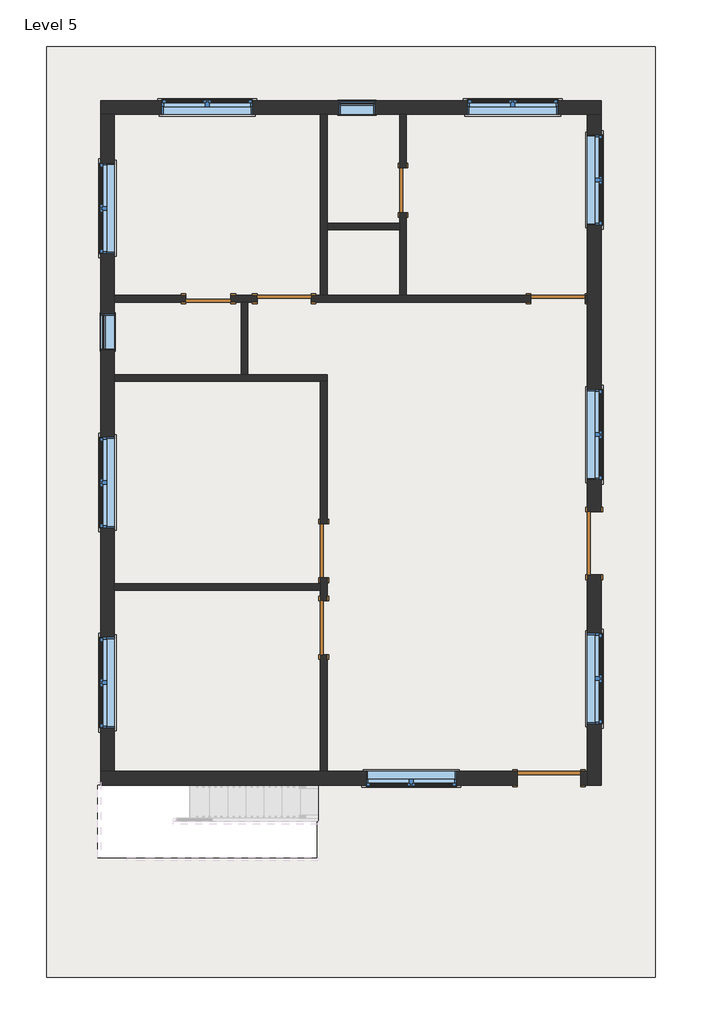
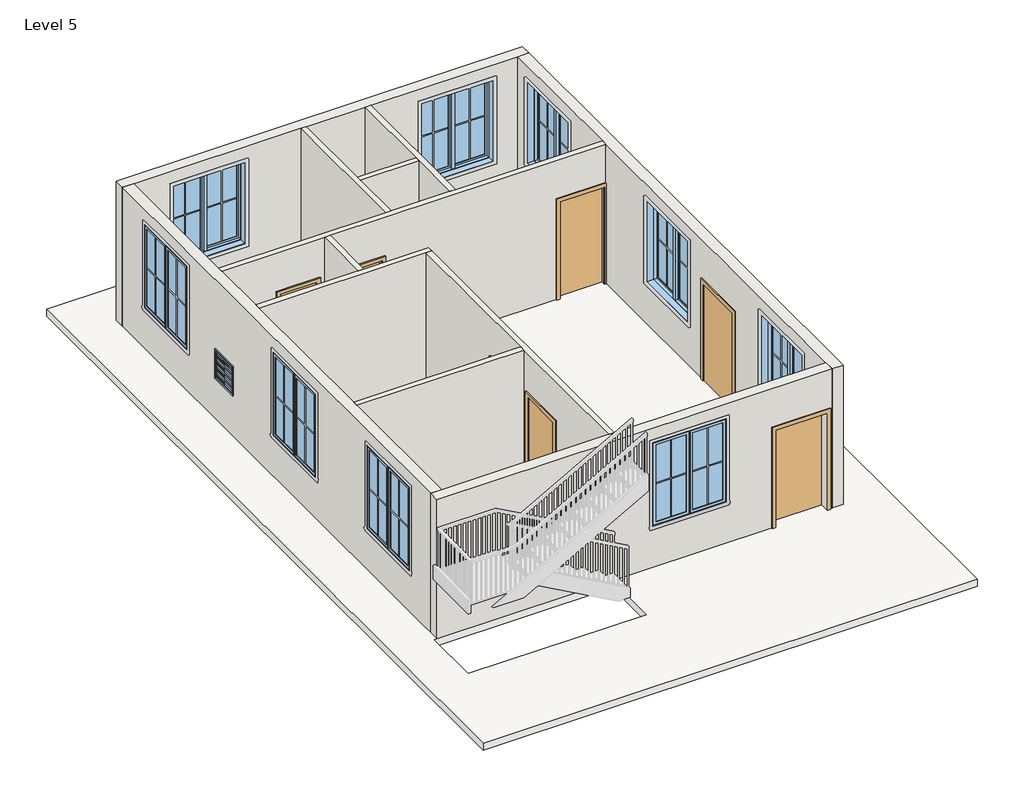
# One storey, part 1 of 3: 12 walls, 11 windows, 8 doors, 1 roof.
"""IFC4 building model written with IfcOpenShell, lengths in millimetres."""

from ifc_helpers import new_model, si_unit, frame, origin, place, context, project, spatial, polyline, outline, extrude, faceted_brep, transform, mapped, element, save
from components import door_78caadf7, single_flush_door_3_e5f9f3c4, single_flush_door_3_305aa2a5, door_9d399b00, door_0848dd25, window_casement_double_win_5_f93960c7, window_f2d8fef0

model = new_model("IFC4")

# Units and contexts
model_context = context("Model", 3, world=origin())
ifc_project = project(units=[si_unit("LENGTHUNIT", "METRE", prefix="MILLI")], contexts=[model_context])

# Site, building, storey
site = spatial("IfcSite", under=ifc_project)
building = spatial("IfcBuilding", under=site)
storey = spatial("IfcBuildingStorey", under=building, Name="Level 5", Elevation=9601.2)

# Doors
placement = place(None, origin())
door_shape = door_78caadf7(model_context)
element("IfcDoor", 1, ObjectType="Single-Flush : DOOR 2'6\"", at=placement, inside=storey, context=model_context, shape_type="MappedRepresentation", body=[
    mapped(door_shape, transform((-377.1698569, 4707.5566963, 9601.2), x_axis=(0.0, -1.0, 0.0), y_axis=(1.0, 0.0, 0.0), z_axis=(0.0, 0.0, 1.0))),
])
element("IfcDoor", 2, ObjectType="Single-Flush : DOOR 2'6\"", at=placement, inside=storey, context=model_context, shape_type="MappedRepresentation", body=[
    mapped(door_shape, transform((-3653.7698569, 2878.7566963, 9601.2), x_axis=(1.0, 0.0, 0.0), y_axis=(0.0, 1.0, 0.0), z_axis=(0.0, 0.0, 1.0))),
])
single_flush_door_3_shape = single_flush_door_3_e5f9f3c4(model_context)
element("IfcDoor", 3, ObjectType="Single-Flush : DOOR 3'", at=placement, inside=storey, context=model_context, shape_type="MappedRepresentation", body=[
    mapped(single_flush_door_3_shape, transform((-2377.4198569, 2878.7566963, 9601.2), x_axis=(1.0, 0.0, 0.0), y_axis=(0.0, 1.0, 0.0), z_axis=(0.0, 0.0, 1.0))),
])
element("IfcDoor", 4, ObjectType="Single-Flush : DOOR 3'", at=placement, inside=storey, context=model_context, shape_type="MappedRepresentation", body=[
    mapped(single_flush_door_3_shape, transform((2232.6801431, 2878.7566963, 9601.2), x_axis=(1.0, 0.0, 0.0), y_axis=(0.0, 1.0, 0.0), z_axis=(0.0, 0.0, 1.0))),
])
element("IfcDoor", 5, ObjectType="Single-Flush : DOOR 3'", at=placement, inside=storey, context=model_context, shape_type="MappedRepresentation", body=[
    mapped(single_flush_door_3_shape, transform((-1710.6698569, -2658.4433037, 9601.2), x_axis=(0.0, 1.0, 0.0), y_axis=(-1.0, 0.0, 0.0), z_axis=(0.0, 0.0, 1.0))),
])
single_flush_door_3_2_shape = single_flush_door_3_305aa2a5(model_context)
element("IfcDoor", 6, ObjectType="Single-Flush : DOOR 3'", at=placement, inside=storey, context=model_context, shape_type="MappedRepresentation", body=[
    mapped(single_flush_door_3_2_shape, transform((-1710.6698569, -1363.0433037, 9601.2), x_axis=(0.0, -1.0, 0.0), y_axis=(1.0, 0.0, 0.0), z_axis=(0.0, 0.0, 1.0))),
])
door_2_shape = door_9d399b00(model_context)
element("IfcDoor", 7, ObjectType="Single-Flush : DOOR 3'6\"", at=placement, inside=storey, context=model_context, shape_type="MappedRepresentation", body=[
    mapped(door_2_shape, transform((2080.2801431, -5192.0933037, 9601.2), x_axis=(1.0, 0.0, 0.0), y_axis=(0.0, 1.0, 0.0), z_axis=(0.0, 0.0, 1.0))),
])
door_3_shape = door_0848dd25(model_context)
element("IfcDoor", 8, ObjectType="Single-Flush : DOOR 3'6\"", at=placement, inside=storey, context=model_context, shape_type="MappedRepresentation", body=[
    mapped(door_3_shape, transform((2842.2801431, -1236.0433037, 9601.2), x_axis=(0.0, -1.0, 0.0), y_axis=(1.0, 0.0, 0.0), z_axis=(0.0, 0.0, 1.0))),
])

# Roof
element("IfcRoof", 9, ObjectType="ROOF 6\"", at=placement, inside=storey, context=model_context, shape_type="SweptSolid", body=[
    extrude(outline(polyline([(-6377.9198569, -8544.8933037), (-6377.9198569, 7126.9066963), (3870.9801431, 7126.9066963), (3870.9801431, -8544.8933037), (-6377.9198569, -8544.8933037)]), holes=[polyline([(-5514.3198569, -5306.3933037), (-5514.3198569, -6525.5933037), (-1831.3198569, -6525.5933037), (-1831.3198569, -5306.3933037), (-5514.3198569, -5306.3933037)])]), frame((0.0, 0.0, 9448.8), z_axis=(0.0, 0.0, 1.0), x_axis=(1.0, 0.0, 0.0)), (0.0, 0.0, 1.0), 152.4),
])

# Walls
element("IfcWall", 10, ObjectType="WALL 4.5\"", at=placement, inside=storey, context=model_context, shape_type="Brep", body=[
    faceted_brep([(2689.8801431, 2821.6066963, 11734.8), (2689.8801431, 2821.6066963, 9601.2), (2727.9801431, 2821.6066963, 9601.2), (2727.9801431, 2821.6066963, 12649.2), (-2987.0198569, 2821.6066963, 12649.2), (-3101.3198569, 2821.6066963, 12649.2), (-5234.9198569, 2821.6066963, 12649.2), (-5234.9198569, 2821.6066963, 9601.2), (-4034.7698569, 2821.6066963, 9601.2), (-4034.7698569, 2821.6066963, 11734.8), (-3272.7698569, 2821.6066963, 11734.8), (-3272.7698569, 2821.6066963, 9601.2), (-3101.3198569, 2821.6066963, 9601.2), (-2987.0198569, 2821.6066963, 9601.2), (-2834.6198569, 2821.6066963, 9601.2), (-2834.6198569, 2821.6066963, 11734.8), (-1920.2198569, 2821.6066963, 11734.8), (-1920.2198569, 2821.6066963, 9601.2), (1775.4801431, 2821.6066963, 9601.2), (1775.4801431, 2821.6066963, 11734.8), (2727.9801431, 2935.9066963, 9601.2), (2689.8801431, 2935.9066963, 9601.2), (2689.8801431, 2935.9066963, 11734.8), (1775.4801431, 2935.9066963, 11734.8), (1775.4801431, 2935.9066963, 9601.2), (-320.0198569, 2935.9066963, 9601.2), (-434.3198569, 2935.9066963, 9601.2), (-1653.5198569, 2935.9066963, 9601.2), (-1767.8198569, 2935.9066963, 9601.2), (-1920.2198569, 2935.9066963, 9601.2), (-1920.2198569, 2935.9066963, 11734.8), (-2834.6198569, 2935.9066963, 11734.8), (-2834.6198569, 2935.9066963, 9601.2), (-3272.7698569, 2935.9066963, 9601.2), (-3272.7698569, 2935.9066963, 11734.8), (-4034.7698569, 2935.9066963, 11734.8), (-4034.7698569, 2935.9066963, 9601.2), (-5234.9198569, 2935.9066963, 9601.2), (-5234.9198569, 2935.9066963, 12649.2), (-1767.8198569, 2935.9066963, 12649.2), (-1653.5198569, 2935.9066963, 12649.2), (-434.3198569, 2935.9066963, 12649.2), (-320.0198569, 2935.9066963, 12649.2), (2727.9801431, 2935.9066963, 12649.2)], [[[0, 1, 2, 3, 4, 5, 6, 7, 8, 9, 10, 11, 12, 13, 14, 15, 16, 17, 18, 19]], [[20, 21, 22, 23, 24, 25, 26, 27, 28, 29, 30, 31, 32, 33, 34, 35, 36, 37, 38, 39, 40, 41, 42, 43]], [[8, 7, 37, 36]], [[14, 13, 12, 11, 33, 32]], [[18, 17, 29, 28, 27, 26, 25, 24]], [[2, 1, 21, 20]], [[3, 2, 20, 43]], [[7, 6, 38, 37]], [[34, 33, 11, 10]], [[35, 34, 10, 9]], [[36, 35, 9, 8]], [[30, 29, 17, 16]], [[31, 30, 16, 15]], [[32, 31, 15, 14]], [[22, 21, 1, 0]], [[23, 22, 0, 19]], [[24, 23, 19, 18]], [[6, 5, 4, 3, 43, 42, 41, 40, 39, 38]]]),
])
element("IfcWall", 11, ObjectType="WALL 4.5\"", at=placement, inside=storey, context=model_context, shape_type="Brep", body=[
    faceted_brep([(-1767.8198569, 5983.9066963, 9601.2), (-1767.8198569, 2935.9066963, 9601.2), (-1767.8198569, 2935.9066963, 12649.2), (-1767.8198569, 5983.9066963, 12649.2), (-1653.5198569, 5983.9066963, 9601.2), (-1653.5198569, 5983.9066963, 12649.2), (-1653.5198569, 4155.1066963, 12649.2), (-1653.5198569, 4040.8066963, 12649.2), (-1653.5198569, 2935.9066963, 12649.2), (-1653.5198569, 2935.9066963, 9601.2), (-1653.5198569, 4040.8066963, 9601.2), (-1653.5198569, 4155.1066963, 9601.2)], [[[0, 1, 2, 3]], [[4, 5, 6, 7, 8, 9, 10, 11]], [[1, 0, 4, 11, 10, 9]], [[0, 3, 5, 4]], [[2, 1, 9, 8]], [[3, 2, 8, 7, 6, 5]]]),
])
element("IfcWall", 12, ObjectType="WALL 4.5\"", at=placement, inside=storey, context=model_context, shape_type="Brep", body=[
    faceted_brep([(-320.0198569, 2935.9066963, 9601.2), (-320.0198569, 4326.5566963, 9601.2), (-320.0198569, 4326.5566963, 11734.8), (-320.0198569, 5088.5566963, 11734.8), (-320.0198569, 5088.5566963, 9601.2), (-320.0198569, 5983.9066963, 9601.2), (-320.0198569, 5983.9066963, 12649.2), (-320.0198569, 2935.9066963, 12649.2), (-434.3198569, 4326.5566963, 11734.8), (-434.3198569, 4326.5566963, 9601.2), (-434.3198569, 4155.1066963, 9601.2), (-434.3198569, 4040.8066963, 9601.2), (-434.3198569, 2935.9066963, 9601.2), (-434.3198569, 2935.9066963, 12649.2), (-434.3198569, 4040.8066963, 12649.2), (-434.3198569, 4155.1066963, 12649.2), (-434.3198569, 5983.9066963, 12649.2), (-434.3198569, 5983.9066963, 9601.2), (-434.3198569, 5088.5566963, 9601.2), (-434.3198569, 5088.5566963, 11734.8)], [[[0, 1, 2, 3, 4, 5, 6, 7]], [[8, 9, 10, 11, 12, 13, 14, 15, 16, 17, 18, 19]], [[18, 17, 5, 4]], [[12, 11, 10, 9, 1, 0]], [[6, 5, 17, 16]], [[0, 7, 13, 12]], [[2, 1, 9, 8]], [[3, 2, 8, 19]], [[4, 3, 19, 18]], [[7, 6, 16, 15, 14, 13]]]),
])
element("IfcWall", 13, ObjectType="WALL 4.5\"", at=placement, inside=storey, context=model_context, shape_type="SweptSolid", body=[
    extrude(outline(polyline([(-434.3198569, 4040.8066963), (-1653.5198569, 4040.8066963), (-1653.5198569, 4155.1066963), (-434.3198569, 4155.1066963), (-434.3198569, 4040.8066963)])), frame((0.0, 0.0, 9601.2), z_axis=(0.0, 0.0, 1.0), x_axis=(1.0, 0.0, 0.0)), (0.0, 0.0, 1.0), 3048.0),
])
element("IfcWall", 14, ObjectType="WALL 4.5\"", at=placement, inside=storey, context=model_context, shape_type="Brep", body=[
    faceted_brep([(-5234.9198569, 1488.1066963, 9601.2), (-1767.8198569, 1488.1066963, 9601.2), (-1653.5198569, 1488.1066963, 9601.2), (-1653.5198569, 1488.1066963, 12649.2), (-1767.8198569, 1488.1066963, 12649.2), (-5234.9198569, 1488.1066963, 12649.2), (-5234.9198569, 1602.4066963, 9601.2), (-5234.9198569, 1602.4066963, 12649.2), (-3101.3198569, 1602.4066963, 12649.2), (-2987.0198569, 1602.4066963, 12649.2), (-1653.5198569, 1602.4066963, 12649.2), (-1653.5198569, 1602.4066963, 9601.2), (-2987.0198569, 1602.4066963, 9601.2), (-3101.3198569, 1602.4066963, 9601.2)], [[[0, 1, 2, 3, 4, 5]], [[6, 7, 8, 9, 10, 11, 12, 13]], [[2, 1, 0, 6, 13, 12, 11]], [[0, 5, 7, 6]], [[3, 2, 11, 10]], [[5, 4, 3, 10, 9, 8, 7]]]),
])
element("IfcWall", 15, ObjectType="WALL 4.5\"", at=placement, inside=storey, context=model_context, shape_type="Brep", body=[
    faceted_brep([(-1767.8198569, -1820.2433037, 9601.2), (-1767.8198569, -1915.4933037, 9601.2), (-1767.8198569, -2029.7933037, 9601.2), (-1767.8198569, -2201.2433037, 9601.2), (-1767.8198569, -2201.2433037, 11734.8), (-1767.8198569, -3115.6433037, 11734.8), (-1767.8198569, -3115.6433037, 9601.2), (-1767.8198569, -5077.7933037, 9601.2), (-1767.8198569, -5077.7933037, 12649.2), (-1767.8198569, -2029.7933037, 12649.2), (-1767.8198569, -1915.4933037, 12649.2), (-1767.8198569, 1488.1066963, 12649.2), (-1767.8198569, 1488.1066963, 9601.2), (-1767.8198569, -905.8433037, 9601.2), (-1767.8198569, -905.8433037, 11734.8), (-1767.8198569, -1820.2433037, 11734.8), (-1653.5198569, -2201.2433037, 11734.8), (-1653.5198569, -2201.2433037, 9601.2), (-1653.5198569, -1820.2433037, 9601.2), (-1653.5198569, -1820.2433037, 11734.8), (-1653.5198569, -905.8433037, 11734.8), (-1653.5198569, -905.8433037, 9601.2), (-1653.5198569, 1488.1066963, 9601.2), (-1653.5198569, 1488.1066963, 12649.2), (-1653.5198569, -5077.7933037, 12649.2), (-1653.5198569, -5077.7933037, 9601.2), (-1653.5198569, -3115.6433037, 9601.2), (-1653.5198569, -3115.6433037, 11734.8)], [[[0, 1, 2, 3, 4, 5, 6, 7, 8, 9, 10, 11, 12, 13, 14, 15]], [[16, 17, 18, 19, 20, 21, 22, 23, 24, 25, 26, 27]], [[13, 12, 22, 21]], [[26, 25, 7, 6]], [[18, 17, 3, 2, 1, 0]], [[12, 11, 23, 22]], [[8, 7, 25, 24]], [[19, 18, 0, 15]], [[20, 19, 15, 14]], [[21, 20, 14, 13]], [[4, 3, 17, 16]], [[5, 4, 16, 27]], [[6, 5, 27, 26]], [[11, 10, 9, 8, 24, 23]]]),
])
element("IfcWall", 16, ObjectType="WALL 4.5\"", at=placement, inside=storey, context=model_context, shape_type="SweptSolid", body=[
    extrude(outline(polyline([(-1767.8198569, -2029.7933037), (-5234.9198569, -2029.7933037), (-5234.9198569, -1915.4933037), (-1767.8198569, -1915.4933037), (-1767.8198569, -2029.7933037)])), frame((0.0, 0.0, 9601.2), z_axis=(0.0, 0.0, 1.0), x_axis=(1.0, 0.0, 0.0)), (0.0, 0.0, 1.0), 3048.0),
])
element("IfcWall", 17, ObjectType="WALL 4.5\"", at=placement, inside=storey, context=model_context, shape_type="SweptSolid", body=[
    extrude(outline(polyline([(-3101.3198569, 1602.4066963), (-3101.3198569, 2821.6066963), (-2987.0198569, 2821.6066963), (-2987.0198569, 1602.4066963), (-3101.3198569, 1602.4066963)])), frame((0.0, 0.0, 9601.2), z_axis=(0.0, 0.0, 1.0), x_axis=(1.0, 0.0, 0.0)), (0.0, 0.0, 1.0), 3048.0),
])
element("IfcWall", 18, ObjectType="WALL 9\"", at=placement, inside=storey, context=model_context, shape_type="Brep", body=[
    faceted_brep([(-5463.5198569, 5983.9066963, 9601.2), (-5234.9198569, 5983.9066963, 9601.2), (-1767.8198569, 5983.9066963, 9601.2), (-1653.5198569, 5983.9066963, 9601.2), (-434.3198569, 5983.9066963, 9601.2), (-320.0198569, 5983.9066963, 9601.2), (2727.9801431, 5983.9066963, 9601.2), (2956.5801431, 5983.9066963, 9601.2), (2956.5801431, 5983.9066963, 12649.2), (2727.9801431, 5983.9066963, 12649.2), (-320.0198569, 5983.9066963, 12649.2), (-434.3198569, 5983.9066963, 12649.2), (-1653.5198569, 5983.9066963, 12649.2), (-1767.8198569, 5983.9066963, 12649.2), (-5234.9198569, 5983.9066963, 12649.2), (-5463.5198569, 5983.9066963, 12649.2), (2232.6801431, 5983.9066963, 12344.4), (2232.6801431, 5983.9066963, 10515.6), (708.6801431, 5983.9066963, 10515.6), (708.6801431, 5983.9066963, 12344.4), (-2910.8198569, 5983.9066963, 12344.4), (-2910.8198569, 5983.9066963, 10515.6), (-4434.8198569, 5983.9066963, 10515.6), (-4434.8198569, 5983.9066963, 12344.4), (-1456.6698569, 5983.9066963, 11125.2), (-847.0698569, 5983.9066963, 11125.2), (-847.0698569, 5983.9066963, 10515.6), (-1456.6698569, 5983.9066963, 10515.6), (-5463.5198569, 6212.5066963, 9601.2), (-5463.5198569, 6212.5066963, 12649.2), (2956.5801431, 6212.5066963, 12649.2), (2956.5801431, 6212.5066963, 9601.2), (2232.6801431, 6212.5066963, 12344.4), (708.6801431, 6212.5066963, 12344.4), (708.6801431, 6212.5066963, 10515.6), (2232.6801431, 6212.5066963, 10515.6), (-2910.8198569, 6212.5066963, 12344.4), (-4434.8198569, 6212.5066963, 12344.4), (-4434.8198569, 6212.5066963, 10515.6), (-2910.8198569, 6212.5066963, 10515.6), (-1456.6698569, 6212.5066963, 11125.2), (-1456.6698569, 6212.5066963, 10515.6), (-847.0698569, 6212.5066963, 10515.6), (-847.0698569, 6212.5066963, 11125.2)], [[[0, 1, 2, 3, 4, 5, 6, 7, 8, 9, 10, 11, 12, 13, 14, 15], [16, 17, 18, 19], [20, 21, 22, 23], [24, 25, 26, 27]], [[28, 29, 30, 31], [32, 33, 34, 35], [36, 37, 38, 39], [40, 41, 42, 43]], [[7, 6, 5, 4, 3, 2, 1, 0, 28, 31]], [[8, 7, 31, 30]], [[0, 15, 29, 28]], [[17, 16, 32, 35]], [[18, 17, 35, 34]], [[19, 18, 34, 33]], [[16, 19, 33, 32]], [[21, 20, 36, 39]], [[22, 21, 39, 38]], [[23, 22, 38, 37]], [[20, 23, 37, 36]], [[41, 40, 24, 27]], [[42, 41, 27, 26]], [[43, 42, 26, 25]], [[40, 43, 25, 24]], [[15, 14, 13, 12, 11, 10, 9, 8, 30, 29]]]),
])
element("IfcWall", 19, ObjectType="WALL 9\"", at=placement, inside=storey, context=model_context, shape_type="Brep", body=[
    faceted_brep([(2727.9801431, -1769.4433037, 11734.8), (2727.9801431, -1769.4433037, 9601.2), (2727.9801431, -5077.7933037, 9601.2), (2727.9801431, -5306.3933037, 9601.2), (2727.9801431, -5306.3933037, 12649.2), (2727.9801431, -5077.7933037, 12649.2), (2727.9801431, 2821.6066963, 12649.2), (2727.9801431, 2935.9066963, 12649.2), (2727.9801431, 5983.9066963, 12649.2), (2727.9801431, 5983.9066963, 9601.2), (2727.9801431, 2935.9066963, 9601.2), (2727.9801431, 2821.6066963, 9601.2), (2727.9801431, -702.6433037, 9601.2), (2727.9801431, -702.6433037, 11734.8), (2727.9801431, 4117.0066963, 12344.4), (2727.9801431, 4117.0066963, 10515.6), (2727.9801431, 5641.0066963, 10515.6), (2727.9801431, 5641.0066963, 12344.4), (2727.9801431, -169.2433037, 12344.4), (2727.9801431, -169.2433037, 10515.6), (2727.9801431, 1354.7566963, 10515.6), (2727.9801431, 1354.7566963, 12344.4), (2727.9801431, -4277.6933037, 12344.4), (2727.9801431, -4277.6933037, 10515.6), (2727.9801431, -2753.6933037, 10515.6), (2727.9801431, -2753.6933037, 12344.4), (2956.5801431, -5306.3933037, 9601.2), (2956.5801431, -1769.4433037, 9601.2), (2956.5801431, -1769.4433037, 11734.8), (2956.5801431, -702.6433037, 11734.8), (2956.5801431, -702.6433037, 9601.2), (2956.5801431, 5983.9066963, 9601.2), (2956.5801431, 5983.9066963, 12649.2), (2956.5801431, -5306.3933037, 12649.2), (2956.5801431, 4117.0066963, 12344.4), (2956.5801431, 5641.0066963, 12344.4), (2956.5801431, 5641.0066963, 10515.6), (2956.5801431, 4117.0066963, 10515.6), (2956.5801431, -169.2433037, 12344.4), (2956.5801431, 1354.7566963, 12344.4), (2956.5801431, 1354.7566963, 10515.6), (2956.5801431, -169.2433037, 10515.6), (2956.5801431, -4277.6933037, 12344.4), (2956.5801431, -2753.6933037, 12344.4), (2956.5801431, -2753.6933037, 10515.6), (2956.5801431, -4277.6933037, 10515.6)], [[[0, 1, 2, 3, 4, 5, 6, 7, 8, 9, 10, 11, 12, 13], [14, 15, 16, 17], [18, 19, 20, 21], [22, 23, 24, 25]], [[26, 27, 28, 29, 30, 31, 32, 33], [34, 35, 36, 37], [38, 39, 40, 41], [42, 43, 44, 45]], [[3, 2, 1, 27, 26]], [[12, 11, 10, 9, 31, 30]], [[9, 8, 32, 31]], [[4, 3, 26, 33]], [[15, 14, 34, 37]], [[16, 15, 37, 36]], [[17, 16, 36, 35]], [[14, 17, 35, 34]], [[19, 18, 38, 41]], [[20, 19, 41, 40]], [[21, 20, 40, 39]], [[18, 21, 39, 38]], [[23, 22, 42, 45]], [[24, 23, 45, 44]], [[25, 24, 44, 43]], [[22, 25, 43, 42]], [[28, 27, 1, 0]], [[29, 28, 0, 13]], [[30, 29, 13, 12]], [[8, 7, 6, 5, 4, 33, 32]]]),
])
element("IfcWall", 20, ObjectType="WALL 9\"", at=placement, inside=storey, context=model_context, shape_type="Brep", body=[
    faceted_brep([(2727.9801431, -5077.7933037, 9601.2), (2613.6801431, -5077.7933037, 9601.2), (2613.6801431, -5077.7933037, 11734.8), (1546.8801431, -5077.7933037, 11734.8), (1546.8801431, -5077.7933037, 9601.2), (-1653.5198569, -5077.7933037, 9601.2), (-1767.8198569, -5077.7933037, 9601.2), (-5234.9198569, -5077.7933037, 9601.2), (-5463.5198569, -5077.7933037, 9601.2), (-5463.5198569, -5077.7933037, 12649.2), (-5234.9198569, -5077.7933037, 12649.2), (-1767.8198569, -5077.7933037, 12649.2), (-1653.5198569, -5077.7933037, 12649.2), (2727.9801431, -5077.7933037, 12649.2), (-999.4698569, -5077.7933037, 12344.4), (-999.4698569, -5077.7933037, 10515.6), (524.5301431, -5077.7933037, 10515.6), (524.5301431, -5077.7933037, 12344.4), (2613.6801431, -5306.3933037, 11734.8), (2613.6801431, -5306.3933037, 9601.2), (2727.9801431, -5306.3933037, 9601.2), (2727.9801431, -5306.3933037, 12649.2), (-1831.3198569, -5306.3933037, 12649.2), (-5463.5198569, -5306.3933037, 12649.2), (-5463.5198569, -5306.3933037, 9601.2), (1546.8801431, -5306.3933037, 9601.2), (1546.8801431, -5306.3933037, 11734.8), (-999.4698569, -5306.3933037, 12344.4), (524.5301431, -5306.3933037, 12344.4), (524.5301431, -5306.3933037, 10515.6), (-999.4698569, -5306.3933037, 10515.6)], [[[0, 1, 2, 3, 4, 5, 6, 7, 8, 9, 10, 11, 12, 13], [14, 15, 16, 17]], [[18, 19, 20, 21, 22, 23, 24, 25, 26], [27, 28, 29, 30]], [[25, 24, 8, 7, 6, 5, 4]], [[20, 19, 1, 0]], [[0, 13, 21, 20]], [[9, 8, 24, 23]], [[15, 14, 27, 30]], [[16, 15, 30, 29]], [[17, 16, 29, 28]], [[14, 17, 28, 27]], [[2, 1, 19, 18]], [[3, 2, 18, 26]], [[4, 3, 26, 25]], [[13, 12, 11, 10, 9, 23, 22, 21]]]),
])
element("IfcWall", 21, ObjectType="WALL 9\"", at=placement, inside=storey, context=model_context, shape_type="Brep", body=[
    faceted_brep([(-5234.9198569, -5077.7933037, 9601.2), (-5234.9198569, -2029.7933037, 9601.2), (-5234.9198569, -1915.4933037, 9601.2), (-5234.9198569, 1488.1066963, 9601.2), (-5234.9198569, 1602.4066963, 9601.2), (-5234.9198569, 2821.6066963, 9601.2), (-5234.9198569, 2935.9066963, 9601.2), (-5234.9198569, 5983.9066963, 9601.2), (-5234.9198569, 5983.9066963, 12649.2), (-5234.9198569, 2935.9066963, 12649.2), (-5234.9198569, 2821.6066963, 12649.2), (-5234.9198569, 1602.4066963, 12649.2), (-5234.9198569, 1488.1066963, 12649.2), (-5234.9198569, -1915.4933037, 12649.2), (-5234.9198569, -2029.7933037, 12649.2), (-5234.9198569, -5077.7933037, 12649.2), (-5234.9198569, -2820.3683037, 12344.4), (-5234.9198569, -2820.3683037, 10515.6), (-5234.9198569, -4344.3683037, 10515.6), (-5234.9198569, -4344.3683037, 12344.4), (-5234.9198569, 548.3066963, 12344.4), (-5234.9198569, 548.3066963, 10515.6), (-5234.9198569, -975.6933037, 10515.6), (-5234.9198569, -975.6933037, 12344.4), (-5234.9198569, 5164.7566963, 12344.4), (-5234.9198569, 5164.7566963, 10515.6), (-5234.9198569, 3640.7566963, 10515.6), (-5234.9198569, 3640.7566963, 12344.4), (-5234.9198569, 2015.1566963, 11125.2), (-5234.9198569, 2624.7566963, 11125.2), (-5234.9198569, 2624.7566963, 10515.6), (-5234.9198569, 2015.1566963, 10515.6), (-5463.5198569, -5077.7933037, 9601.2), (-5463.5198569, -5077.7933037, 12649.2), (-5463.5198569, 5983.9066963, 12649.2), (-5463.5198569, 5983.9066963, 9601.2), (-5463.5198569, -2820.3683037, 12344.4), (-5463.5198569, -4344.3683037, 12344.4), (-5463.5198569, -4344.3683037, 10515.6), (-5463.5198569, -2820.3683037, 10515.6), (-5463.5198569, 548.3066963, 12344.4), (-5463.5198569, -975.6933037, 12344.4), (-5463.5198569, -975.6933037, 10515.6), (-5463.5198569, 548.3066963, 10515.6), (-5463.5198569, 5164.7566963, 12344.4), (-5463.5198569, 3640.7566963, 12344.4), (-5463.5198569, 3640.7566963, 10515.6), (-5463.5198569, 5164.7566963, 10515.6), (-5463.5198569, 2015.1566963, 11125.2), (-5463.5198569, 2015.1566963, 10515.6), (-5463.5198569, 2624.7566963, 10515.6), (-5463.5198569, 2624.7566963, 11125.2)], [[[0, 1, 2, 3, 4, 5, 6, 7, 8, 9, 10, 11, 12, 13, 14, 15], [16, 17, 18, 19], [20, 21, 22, 23], [24, 25, 26, 27], [28, 29, 30, 31]], [[32, 33, 34, 35], [36, 37, 38, 39], [40, 41, 42, 43], [44, 45, 46, 47], [48, 49, 50, 51]], [[7, 6, 5, 4, 3, 2, 1, 0, 32, 35]], [[8, 7, 35, 34]], [[0, 15, 33, 32]], [[17, 16, 36, 39]], [[18, 17, 39, 38]], [[19, 18, 38, 37]], [[16, 19, 37, 36]], [[21, 20, 40, 43]], [[22, 21, 43, 42]], [[23, 22, 42, 41]], [[20, 23, 41, 40]], [[25, 24, 44, 47]], [[26, 25, 47, 46]], [[27, 26, 46, 45]], [[24, 27, 45, 44]], [[49, 48, 28, 31]], [[50, 49, 31, 30]], [[51, 50, 30, 29]], [[48, 51, 29, 28]], [[15, 14, 13, 12, 11, 10, 9, 8, 34, 33]]]),
])

# Windows
window_casement_double_win_5_shape = window_casement_double_win_5_f93960c7(model_context)
element("IfcWindow", 22, ObjectType="Window-Casement-Double : WIN 5'", at=placement, inside=storey, context=model_context, shape_type="MappedRepresentation", body=[
    mapped(window_casement_double_win_5_shape, transform((-5349.2198569, -3582.3683037, 9601.2), x_axis=(0.0, 1.0, 0.0), y_axis=(-1.0, 0.0, 0.0), z_axis=(0.0, 0.0, 1.0))),
])
element("IfcWindow", 23, ObjectType="Window-Casement-Double : WIN 5'", at=placement, inside=storey, context=model_context, shape_type="MappedRepresentation", body=[
    mapped(window_casement_double_win_5_shape, transform((-5349.2198569, -213.6933037, 9601.2), x_axis=(0.0, 1.0, 0.0), y_axis=(-1.0, 0.0, 0.0), z_axis=(0.0, 0.0, 1.0))),
])
element("IfcWindow", 24, ObjectType="Window-Casement-Double : WIN 5'", at=placement, inside=storey, context=model_context, shape_type="MappedRepresentation", body=[
    mapped(window_casement_double_win_5_shape, transform((-5349.2198569, 4402.7566963, 9601.2), x_axis=(0.0, 1.0, 0.0), y_axis=(-1.0, 0.0, 0.0), z_axis=(0.0, 0.0, 1.0))),
])
element("IfcWindow", 25, ObjectType="Window-Casement-Double : WIN 5'", at=placement, inside=storey, context=model_context, shape_type="MappedRepresentation", body=[
    mapped(window_casement_double_win_5_shape, transform((2842.2801431, 4879.0066963, 9601.2), x_axis=(0.0, -1.0, 0.0), y_axis=(1.0, 0.0, 0.0), z_axis=(0.0, 0.0, 1.0))),
])
element("IfcWindow", 26, ObjectType="Window-Casement-Double : WIN 5'", at=placement, inside=storey, context=model_context, shape_type="MappedRepresentation", body=[
    mapped(window_casement_double_win_5_shape, transform((2842.2801431, 592.7566963, 9601.2), x_axis=(0.0, -1.0, 0.0), y_axis=(1.0, 0.0, 0.0), z_axis=(0.0, 0.0, 1.0))),
])
element("IfcWindow", 27, ObjectType="Window-Casement-Double : WIN 5'", at=placement, inside=storey, context=model_context, shape_type="MappedRepresentation", body=[
    mapped(window_casement_double_win_5_shape, transform((2842.2801431, -3515.6933037, 9601.2), x_axis=(0.0, -1.0, 0.0), y_axis=(1.0, 0.0, 0.0), z_axis=(0.0, 0.0, 1.0))),
])
element("IfcWindow", 28, ObjectType="Window-Casement-Double : WIN 5'", at=placement, inside=storey, context=model_context, shape_type="MappedRepresentation", body=[
    mapped(window_casement_double_win_5_shape, transform((-237.4698569, -5192.0933037, 9601.2), x_axis=(-1.0, 0.0, 0.0), y_axis=(0.0, -1.0, 0.0), z_axis=(0.0, 0.0, 1.0))),
])
element("IfcWindow", 29, ObjectType="Window-Casement-Double : WIN 5'", at=placement, inside=storey, context=model_context, shape_type="MappedRepresentation", body=[
    mapped(window_casement_double_win_5_shape, transform((1470.6801431, 6098.2066963, 9601.2), x_axis=(1.0, 0.0, 0.0), y_axis=(0.0, 1.0, 0.0), z_axis=(0.0, 0.0, 1.0))),
])
element("IfcWindow", 30, ObjectType="Window-Casement-Double : WIN 5'", at=placement, inside=storey, context=model_context, shape_type="MappedRepresentation", body=[
    mapped(window_casement_double_win_5_shape, transform((-3672.8198569, 6098.2066963, 9601.2), x_axis=(1.0, 0.0, 0.0), y_axis=(0.0, 1.0, 0.0), z_axis=(0.0, 0.0, 1.0))),
])
window_shape = window_f2d8fef0(model_context)
element("IfcWindow", 31, ObjectType="Window-Louvers : 24\" x 24\"", at=placement, inside=storey, context=model_context, shape_type="MappedRepresentation", body=[
    mapped(window_shape, transform((-1151.8698569, 6104.5566963, 9601.2), x_axis=(1.0, 0.0, 0.0), y_axis=(0.0, 1.0, 0.0), z_axis=(0.0, 0.0, 1.0))),
])
element("IfcWindow", 32, ObjectType="Window-Louvers : 24\" x 24\"", at=placement, inside=storey, context=model_context, shape_type="MappedRepresentation", body=[
    mapped(window_shape, transform((-5355.5698569, 2319.9566963, 9601.2), x_axis=(0.0, 1.0, 0.0), y_axis=(-1.0, 0.0, 0.0), z_axis=(0.0, 0.0, 1.0))),
])

save(model, "model.ifc")

# Revit data of these elements
# Type "Single-Flush : DOOR 2'6\""
#   Type Mark = "10"
#   Construction Type Id = "MDOOR"
#   Assembly Code = "C1020"
#   Analytic Construction = "Metal"
#   Thickness = 0' - 2"
#   Heat Transfer Coefficient (U) = 0.651978 BTU/(h·ft²·°F)
#   Height = 7' - 0"
#   Trim Projection Ext = 0' - 1"
#   Trim Projection Int = 0' - 1"
#   Trim Width = 0' - 3"
#   Width = 2' - 6"
#   Define Thermal Properties by = 1
#   Door Material = Door - Panel
#   Frame Material = Door - Frame
#   Visual Light Transmittance = 0
#   Solar Heat Gain Coefficient = 0
#   Function = (empty or 0)
#   Wall Closure = (empty or 0)
# Type "Single-Flush : DOOR 3'"
#   Type Mark = "8"
#   Construction Type Id = "MDOOR"
#   Assembly Code = "C1020"
#   Analytic Construction = "Metal"
#   Thickness = 0' - 2"
#   Heat Transfer Coefficient (U) = 0.651978 BTU/(h·ft²·°F)
#   Height = 7' - 0"
#   Trim Projection Ext = 0' - 1"
#   Trim Projection Int = 0' - 1"
#   Trim Width = 0' - 3"
#   Width = 3' - 0"
#   Define Thermal Properties by = 1
#   Door Material = Door - Panel
#   Frame Material = Door - Frame
#   Visual Light Transmittance = 0
#   Solar Heat Gain Coefficient = 0
#   Function = (empty or 0)
#   Wall Closure = (empty or 0)
# Type "Single-Flush : DOOR 3'6\""
#   Type Mark = "9"
#   Construction Type Id = "MDOOR"
#   Assembly Code = "C1020"
#   Analytic Construction = "Metal"
#   Thickness = 0' - 2"
#   Heat Transfer Coefficient (U) = 0.651978 BTU/(h·ft²·°F)
#   Height = 7' - 0"
#   Trim Projection Ext = 0' - 1"
#   Trim Projection Int = 0' - 1"
#   Trim Width = 0' - 3"
#   Width = 3' - 6"
#   Define Thermal Properties by = 1
#   Door Material = Door - Panel
#   Frame Material = Door - Frame
#   Visual Light Transmittance = 0
#   Solar Heat Gain Coefficient = 0
#   Function = (empty or 0)
#   Wall Closure = (empty or 0)
# Type "ROOF 6\""
#   Assembly Code = "B1020"
#   Layers, outside or top first: 0' - 6" no material (function 1)
# Type "WALL 4.5\""
#   Assembly Code = "B2010"
#   Layers, outside or top first: 0' - 4 1/2" no material (function 1)
# Type "WALL 9\""
#   Assembly Code = "B2010"
#   Layers, outside or top first: 0' - 9" no material (function 1)
# Type "Window-Casement-Double : WIN 5'"
#   Type Mark = "20"
#   Fire Rating = "0.5h"
#   Assembly Code = "B2020100"
#   Analytic Construction = "Double glazing - domestic"
#   Frame Extension [instance default] = 0' - 0 1/4"
#   Window Inset [instance default] = 0' - 0"
#   Wall Thickness [instance default] = 0' - 6"
#   Interior Wall Closure [instance default] = 0' - 2 1/4"
#   Half Width = 2' - 6"
#   Visual Light Transmittance = 0.81
#   Thermal Resistance (R) = 1.8146 (h·ft²·°F)/BTU
#   Solar Heat Gain Coefficient = 0.76
#   Rough Width = 5' - 0 1/2"
#   Rough Height = 6' - 0 1/2"
#   Height = 6' - 0"
#   Heat Transfer Coefficient (U) = 0.5511 BTU/(h·ft²·°F)
#   Exterior Wall Closure [instance default] = 0' - 1 1/4"
#   Extension Jamb [instance default] = 0' - 2 1/4"
#   Default Sill Height = 3' - 0"
#   Width = 5' - 0"
#   Muntin Visibility = yes
#   Interior Trim Visibility [instance default] = yes
#   Exterior Trim Visibility [instance default] = yes
#   Extension Jamb Visibility [instance default] = yes
#   Interior Trim Material = Wood - Stained
#   Muntin Pattern = Muntin Pattern_2x2 : Muntin Pattern_2x2
#   Interior Trim = Trim-Window-Interior-Flat : Picture Frame
#   Interior Frame Material = Wood - Stained
#   Glass Panel Material = Glass
#   Exterior Trim Material = Clad - White
#   Exterior Trim = Trim-Window-Exterior-Flat : with Sill
#   Exterior Frame Material = Clad - White
#   Wall Closure = (empty or 0)
# Type "Window-Louvers : 24\" x 24\""
#   Type Mark = "21"
#   Construction Type Id = "GSP4R"
#   Assembly Code = "B20"
#   Analytic Construction = "1/8 in Pilkington single glazing"
#   Visual Light Transmittance = 0.9
#   Thermal Resistance (R) = 1.53941 (h·ft²·°F)/BTU
#   Solar Heat Gain Coefficient = 0.78
#   Max Height = 1' - 11.74264"
#   Height = 2' - 0"
#   Heat Transfer Coefficient (U) = 0.6496 BTU/(h·ft²·°F)
#   Blade Width [instance default] = 1' - 10 1/2"
#   Blade Vertical Thickness = 0' - 0.35355"
#   Blade Thickness = 0' - 0 1/4"
#   Blade Spacing = 0' - 1 1/2"
#   Blade Height = 0' - 1.85355"
#   Blade Depth = 0' - 3"
#   Blade Angle = 45.00°
#   Default Sill Height = 3' - 0"
#   Trim Projection_Exterior = 0' - 0 1/2"
#   Trim Projection_Interior = 0' - 0 1/2"
#   Trim Width_Exterior = 0' - 1 1/2"
#   Trim Width_Interior = 0' - 1 1/2"
#   Width = 2' - 0"
#   Max Blade Count = 12
#   Define Thermal Properties by = 1
#   Blade Count = 12
#   Frame Material = Birch
#   Louver Material = Birch
#   Trim Exterior Material = Birch
#   Trim Interior Material = Birch
#   Wall Closure = (empty or 0)
# Elements 1, 2 (IfcDoor, "Single-Flush : DOOR 2'6\"")
#   Phase Created = New Construction
#   Materials on its faces: "Door - Frame", "Door - Panel"
# Elements 3, 4, 5, 6 (IfcDoor, "Single-Flush : DOOR 3'")
#   Phase Created = New Construction
#   Materials on its faces: "Door - Frame", "Door - Panel"
# Elements 7, 8 (IfcDoor, "Single-Flush : DOOR 3'6\"")
#   Phase Created = New Construction
#   Materials on its faces: "Door - Frame", "Door - Panel"
# Element 9 (IfcRoof, "ROOF 6\"")
#   built-in parameter 1001705 = 31.5 (stored number, unit not read)
#   built-in parameter 1001701 = -0.5 (stored number, unit not read)
#   built-in parameter 1001710 = 33615
#   Phase Created = New Construction
#   Materials on its faces: "Default Roof", "Parking Stripe", "Wood - Stained"
# Elements 10, 11, 12, 13, 14, 15, 16, 17 (IfcWall, "WALL 4.5\"")
#   Top Offset = 0' - 0"
#   Base Offset = 0' - 0"
#   Unconnected Height = 10' - 0"
#   wall height = 10' - 0"
#   Phase Created = New Construction
#   Base Constraint = Level 5
#   Materials on its faces: "Default Wall"
# Elements 18, 19, 20, 21 (IfcWall, "WALL 9\"")
#   Top Offset = 0' - 0"
#   Base Offset = 0' - 0"
#   Unconnected Height = 10' - 0"
#   wall height = 10' - 0"
#   Phase Created = New Construction
#   Base Constraint = Level 5
#   Materials on its faces: "Default Wall", "Cherry"
# Element 22 (IfcWindow, "Window-Casement-Double : WIN 5'")
#   Mark = "34"
#   Window Inset = 0' - 0"
#   Interior Wall Closure = 0' - 2 1/4"
#   Frame Extension = 0' - 0 1/4"
#   Exterior Wall Closure = 0' - 1 1/4"
#   Interior Trim Visibility = yes
#   Exterior Trim Visibility = yes
#   Phase Created = New Construction
#   Materials on its faces: "Wood - Stained", "Glass", "Clad - White"
# Element 23 (IfcWindow, "Window-Casement-Double : WIN 5'")
#   Mark = "35"
#   Window Inset = 0' - 0"
#   Interior Wall Closure = 0' - 2 1/4"
#   Frame Extension = 0' - 0 1/4"
#   Exterior Wall Closure = 0' - 1 1/4"
#   Interior Trim Visibility = yes
#   Exterior Trim Visibility = yes
#   Phase Created = New Construction
#   Materials on its faces: "Wood - Stained", "Glass", "Clad - White"
# Element 24 (IfcWindow, "Window-Casement-Double : WIN 5'")
#   Mark = "36"
#   Window Inset = 0' - 0"
#   Interior Wall Closure = 0' - 2 1/4"
#   Frame Extension = 0' - 0 1/4"
#   Exterior Wall Closure = 0' - 1 1/4"
#   Interior Trim Visibility = yes
#   Exterior Trim Visibility = yes
#   Phase Created = New Construction
#   Materials on its faces: "Wood - Stained", "Glass", "Clad - White"
# Element 25 (IfcWindow, "Window-Casement-Double : WIN 5'")
#   Mark = "37"
#   Window Inset = 0' - 0"
#   Interior Wall Closure = 0' - 2 1/4"
#   Frame Extension = 0' - 0 1/4"
#   Exterior Wall Closure = 0' - 1 1/4"
#   Interior Trim Visibility = yes
#   Exterior Trim Visibility = yes
#   Phase Created = New Construction
#   Materials on its faces: "Wood - Stained", "Glass", "Clad - White"
# Element 26 (IfcWindow, "Window-Casement-Double : WIN 5'")
#   Mark = "38"
#   Window Inset = 0' - 0"
#   Interior Wall Closure = 0' - 2 1/4"
#   Frame Extension = 0' - 0 1/4"
#   Exterior Wall Closure = 0' - 1 1/4"
#   Interior Trim Visibility = yes
#   Exterior Trim Visibility = yes
#   Phase Created = New Construction
#   Materials on its faces: "Wood - Stained", "Glass", "Clad - White"
# Element 27 (IfcWindow, "Window-Casement-Double : WIN 5'")
#   Mark = "39"
#   Window Inset = 0' - 0"
#   Interior Wall Closure = 0' - 2 1/4"
#   Frame Extension = 0' - 0 1/4"
#   Exterior Wall Closure = 0' - 1 1/4"
#   Interior Trim Visibility = yes
#   Exterior Trim Visibility = yes
#   Phase Created = New Construction
#   Materials on its faces: "Wood - Stained", "Glass", "Clad - White"
# Element 28 (IfcWindow, "Window-Casement-Double : WIN 5'")
#   Mark = "40"
#   Window Inset = 0' - 0"
#   Interior Wall Closure = 0' - 2 1/4"
#   Frame Extension = 0' - 0 1/4"
#   Exterior Wall Closure = 0' - 1 1/4"
#   Interior Trim Visibility = yes
#   Exterior Trim Visibility = yes
#   Phase Created = New Construction
#   Materials on its faces: "Wood - Stained", "Glass", "Clad - White"
# Element 29 (IfcWindow, "Window-Casement-Double : WIN 5'")
#   Mark = "41"
#   Window Inset = 0' - 0"
#   Interior Wall Closure = 0' - 2 1/4"
#   Frame Extension = 0' - 0 1/4"
#   Exterior Wall Closure = 0' - 1 1/4"
#   Interior Trim Visibility = yes
#   Exterior Trim Visibility = yes
#   Phase Created = New Construction
#   Materials on its faces: "Wood - Stained", "Glass", "Clad - White"
# Element 30 (IfcWindow, "Window-Casement-Double : WIN 5'")
#   Mark = "42"
#   Window Inset = 0' - 0"
#   Interior Wall Closure = 0' - 2 1/4"
#   Frame Extension = 0' - 0 1/4"
#   Exterior Wall Closure = 0' - 1 1/4"
#   Interior Trim Visibility = yes
#   Exterior Trim Visibility = yes
#   Phase Created = New Construction
#   Materials on its faces: "Wood - Stained", "Glass", "Clad - White"
# Element 31 (IfcWindow, "Window-Louvers : 24\" x 24\"")
#   Mark = "43"
#   Blade Width = 1' - 10 1/2"
#   Phase Created = New Construction
#   Materials on its faces: "Birch"
# Element 32 (IfcWindow, "Window-Louvers : 24\" x 24\"")
#   Mark = "44"
#   Blade Width = 1' - 10 1/2"
#   Phase Created = New Construction
#   Materials on its faces: "Birch"
# Materials
#   "Door - Panel": class "Wood", colour RGB 210 159 95, transparency 0, Cost = 0
#   "Door - Frame": colour RGB 118 70 51, transparency 0, Cost = 0
#   "Wood - Stained": class "Wood", colour RGB 224 178 126, transparency 0, Cost = 0
#   "Glass": class "Glass", colour RGB 0 128 192, transparency 0.75, Description = "Soda Lime Glass", Cost = 0
#   "Clad - White": class "Wood", colour RGB 242 242 238, transparency 0, Cost = 0
#   "Birch": class "Wood", colour RGB 224 178 126, transparency 0, Description = "Betula Alleghaniensis", Cost = 0
#   "Default Roof": colour RGB 88 101 114, transparency 0, Cost = 0
#   "Parking Stripe": class "Paint", colour RGB 250 250 91, transparency 0, Cost = 0
#   "Default Wall": colour RGB 128 128 128, transparency 0, Cost = 0
#   "Cherry": class "Wood", colour RGB 226 177 128, transparency 0, Description = "Prunus Serotina", Cost = 0
